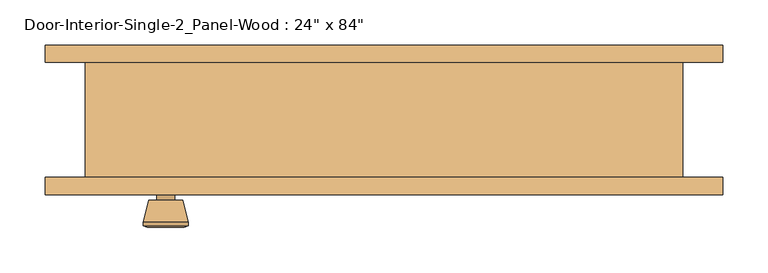
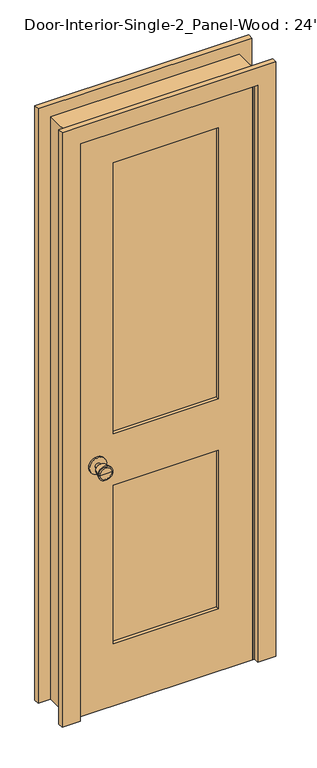
"""IFC4 building model written with IfcOpenShell, lengths in millimetres: door geometry."""

from ifc_helpers import new_model, si_unit, point, frame, frame_2d, origin, place, context, project, spatial, polyline, circle_curve, trimmed, segment, composite_curve, outline, extrude, faceted_brep, source, transform, mapped, element, save
from ifc_brep_helpers import plane_surface, cylinder_surface, revolved_surface, advanced_brep


def door_e337afa5(model_context):
    return source(origin(), model_context, "Body", "SolidModel", [
        advanced_brep(
        [(-241.3, -19.4, 914.4), (-251.3, -19.4, 914.4), (-231.3, -19.4, 914.4), (-220.8241324, 29.6, 914.4), (-261.7758676, 29.6, 914.4), (-241.3, 29.6, 914.4), (-216.3, 27.7721319, 914.4), (-266.3, 27.7721319, 914.4), (-216.3, 24.3084537, 914.4), (-266.3, 24.3084537, 914.4), (-222.663764, -0.4, 914.4), (-259.936236, -0.4, 914.4), (-231.3, -0.4, 914.4), (-251.3, -0.4, 914.4)],
        [
            (0, 1),
            (1, 2, circle_curve(frame((-241.3, -19.4, 914.4), z_axis=(0.0, -1.0, 0.0), x_axis=(-1.0, 0.0, 0.0)), 10.0)),
            (2, 0),
            (2, 1, circle_curve(frame((-241.3, -19.4, 914.4), z_axis=(0.0, -1.0, 0.0), x_axis=(-1.0, 0.0, 0.0)), 10.0)),
            (3, 4, circle_curve(frame((-241.3, 29.6, 914.4), z_axis=(0.0, 1.0, 0.0), x_axis=(-1.0, 0.0, 0.0)), 20.4758676)),
            (4, 5),
            (5, 3),
            (4, 3, circle_curve(frame((-241.3, 29.6, 914.4), z_axis=(0.0, 1.0, 0.0), x_axis=(-1.0, 0.0, 0.0)), 20.4758676)),
            (6, 7, circle_curve(frame((-241.3, 27.7721319, 914.4), z_axis=(0.0, 1.0, 0.0), x_axis=(-1.0, 0.0, 0.0)), 25.0)),
            (7, 4),
            (3, 6),
            (7, 6, circle_curve(frame((-241.3, 27.7721319, 914.4), z_axis=(0.0, 1.0, 0.0), x_axis=(-1.0, 0.0, 0.0)), 25.0)),
            (8, 9, circle_curve(frame((-241.3, 24.3084537, 914.4), z_axis=(0.0, 1.0, 0.0), x_axis=(-1.0, 0.0, 0.0)), 25.0)),
            (9, 7),
            (6, 8),
            (9, 8, circle_curve(frame((-241.3, 24.3084537, 914.4), z_axis=(0.0, 1.0, 0.0), x_axis=(-1.0, 0.0, 0.0)), 25.0)),
            (10, 11, circle_curve(frame((-241.3, -0.4, 914.4), z_axis=(0.0, 1.0, 0.0), x_axis=(-1.0, 0.0, 0.0)), 18.636236)),
            (11, 9),
            (8, 10),
            (11, 10, circle_curve(frame((-241.3, -0.4, 914.4), z_axis=(0.0, 1.0, 0.0), x_axis=(-1.0, 0.0, 0.0)), 18.636236)),
            (12, 13, circle_curve(frame((-241.3, -0.4, 914.4), z_axis=(0.0, 1.0, 0.0), x_axis=(-1.0, 0.0, 0.0)), 10.0)),
            (13, 11),
            (10, 12),
            (13, 12, circle_curve(frame((-241.3, -0.4, 914.4), z_axis=(0.0, 1.0, 0.0), x_axis=(-1.0, 0.0, 0.0)), 10.0)),
            (1, 13),
            (12, 2),
        ],
        [
            plane_surface(frame((-241.3, -19.4, 914.4), z_axis=(0.0, -1.0, 0.0), x_axis=(-1.0, 0.0, 0.0))),
            plane_surface(frame((-241.3, 29.6, 914.4), z_axis=(0.0, 1.0, 0.0), x_axis=(-1.0, 0.0, 0.0))),
            revolved_surface(polyline([(-261.7758676, 29.6, 914.4), (-266.3, 27.7721319, 914.4)]), (-241.3, -19.4, 914.4), (0.0, -1.0, 0.0)),
            cylinder_surface(frame((-241.3, -19.4, 914.4), z_axis=(0.0, -1.0, 0.0), x_axis=(-1.0, 0.0, 0.0)), 25.0),
            revolved_surface(polyline([(-266.3, 24.3084537, 914.4), (-259.936236, -0.4, 914.4)]), (-241.3, -19.4, 914.4), (0.0, -1.0, 0.0)),
            plane_surface(frame((-241.3, -0.4, 914.4), z_axis=(0.0, -1.0, 0.0), x_axis=(-1.0, 0.0, 0.0))),
            cylinder_surface(frame((-241.3, -19.4, 914.4), z_axis=(0.0, -1.0, 0.0), x_axis=(-1.0, 0.0, 0.0)), 10.0),
        ],
        [
            (0, [[1, 2, 3]]),
            (0, [[-3, 4, -1]]),
            (1, [[5, 6, 7]]),
            (1, [[8, -7, -6]]),
            (2, [[9, 10, -5, 11]]),
            (2, [[12, -11, -8, -10]]),
            (3, [[13, 14, -9, 15]]),
            (3, [[16, -15, -12, -14]]),
            (4, [[17, 18, -13, 19]]),
            (4, [[20, -19, -16, -18]]),
            (5, [[21, 22, -17, 23]]),
            (5, [[24, -23, -20, -22]]),
            (6, [[-2, 25, -21, 26]]),
            (6, [[-4, -26, -24, -25]]),
        ],
    ),
        extrude(outline(composite_curve([segment(trimmed(circle_curve(frame_2d((914.4, -241.3)), 30.0), [point((914.4, -271.3))], [point((914.4, -211.3))], False, "CARTESIAN"), True, "CONTINUOUS"), segment(trimmed(circle_curve(frame_2d((914.4, -241.3)), 30.0), [point((914.4, -211.3))], [point((914.4, -271.3))], False, "CARTESIAN"), True, "CONTINUOUS")], self_intersect=False)), frame((0.0, -25.4, 0.0), z_axis=(0.0, 1.0, 0.0), x_axis=(0.0, 0.0, 1.0)), (0.0, 0.0, 1.0), 6.0),
        advanced_brep(
        [(-241.3, -66.325, 914.4), (-231.3, -66.325, 914.4), (-251.3, -66.325, 914.4), (-220.8241324, -115.325, 914.4), (-241.3, -115.325, 914.4), (-261.7758676, -115.325, 914.4), (-216.3, -113.4971319, 914.4), (-266.3, -113.4971319, 914.4), (-216.3, -110.0334537, 914.4), (-266.3, -110.0334537, 914.4), (-222.663764, -85.325, 914.4), (-259.936236, -85.325, 914.4), (-231.3, -85.325, 914.4), (-251.3, -85.325, 914.4)],
        [
            (0, 1),
            (1, 2, circle_curve(frame((-241.3, -66.325, 914.4), z_axis=(0.0, 1.0, 0.0), x_axis=(-1.0, 0.0, 0.0)), 10.0)),
            (2, 0),
            (2, 1, circle_curve(frame((-241.3, -66.325, 914.4), z_axis=(0.0, 1.0, 0.0), x_axis=(-1.0, 0.0, 0.0)), 10.0)),
            (3, 4),
            (4, 5),
            (5, 3, circle_curve(frame((-241.3, -115.325, 914.4), z_axis=(0.0, -1.0, 0.0), x_axis=(-1.0, 0.0, 0.0)), 20.4758676)),
            (3, 5, circle_curve(frame((-241.3, -115.325, 914.4), z_axis=(0.0, -1.0, 0.0), x_axis=(-1.0, 0.0, 0.0)), 20.4758676)),
            (6, 3),
            (5, 7),
            (7, 6, circle_curve(frame((-241.3, -113.4971319, 914.4), z_axis=(0.0, -1.0, 0.0), x_axis=(-1.0, 0.0, 0.0)), 25.0)),
            (6, 7, circle_curve(frame((-241.3, -113.4971319, 914.4), z_axis=(0.0, -1.0, 0.0), x_axis=(-1.0, 0.0, 0.0)), 25.0)),
            (8, 6),
            (7, 9),
            (9, 8, circle_curve(frame((-241.3, -110.0334537, 914.4), z_axis=(0.0, -1.0, 0.0), x_axis=(-1.0, 0.0, 0.0)), 25.0)),
            (8, 9, circle_curve(frame((-241.3, -110.0334537, 914.4), z_axis=(0.0, -1.0, 0.0), x_axis=(-1.0, 0.0, 0.0)), 25.0)),
            (10, 8),
            (9, 11),
            (11, 10, circle_curve(frame((-241.3, -85.325, 914.4), z_axis=(0.0, -1.0, 0.0), x_axis=(-1.0, 0.0, 0.0)), 18.636236)),
            (10, 11, circle_curve(frame((-241.3, -85.325, 914.4), z_axis=(0.0, -1.0, 0.0), x_axis=(-1.0, 0.0, 0.0)), 18.636236)),
            (12, 10),
            (11, 13),
            (13, 12, circle_curve(frame((-241.3, -85.325, 914.4), z_axis=(0.0, -1.0, 0.0), x_axis=(-1.0, 0.0, 0.0)), 10.0)),
            (12, 13, circle_curve(frame((-241.3, -85.325, 914.4), z_axis=(0.0, -1.0, 0.0), x_axis=(-1.0, 0.0, 0.0)), 10.0)),
            (1, 12),
            (13, 2),
        ],
        [
            plane_surface(frame((-241.3, -66.325, 914.4), z_axis=(0.0, 1.0, 0.0), x_axis=(-1.0, 0.0, 0.0))),
            plane_surface(frame((-241.3, -115.325, 914.4), z_axis=(0.0, -1.0, 0.0), x_axis=(-1.0, 0.0, 0.0))),
            revolved_surface(polyline([(-261.7758676, -115.325, 914.4), (-266.3, -113.4971319, 914.4)]), (-241.3, -66.325, 914.4), (0.0, 1.0, 0.0)),
            cylinder_surface(frame((-241.3, -66.325, 914.4), z_axis=(0.0, 1.0, 0.0), x_axis=(-1.0, 0.0, 0.0)), 25.0),
            revolved_surface(polyline([(-266.3, -110.0334537, 914.4), (-259.936236, -85.325, 914.4)]), (-241.3, -66.325, 914.4), (0.0, 1.0, 0.0)),
            plane_surface(frame((-241.3, -85.325, 914.4), z_axis=(0.0, 1.0, 0.0), x_axis=(-1.0, 0.0, 0.0))),
            cylinder_surface(frame((-241.3, -66.325, 914.4), z_axis=(0.0, 1.0, 0.0), x_axis=(-1.0, 0.0, 0.0)), 10.0),
        ],
        [
            (0, [[1, 2, 3]]),
            (0, [[-3, 4, -1]]),
            (1, [[5, 6, 7]]),
            (1, [[-6, -5, 8]]),
            (2, [[9, -7, 10, 11]]),
            (2, [[-10, -8, -9, 12]]),
            (3, [[13, -11, 14, 15]]),
            (3, [[-14, -12, -13, 16]]),
            (4, [[17, -15, 18, 19]]),
            (4, [[-18, -16, -17, 20]]),
            (5, [[21, -19, 22, 23]]),
            (5, [[-22, -20, -21, 24]]),
            (6, [[25, -23, 26, -2]]),
            (6, [[-26, -24, -25, -4]]),
        ],
    ),
        extrude(outline(composite_curve([segment(trimmed(circle_curve(frame_2d((914.4, -241.3)), 30.0), [point((914.4, -271.3))], [point((914.4, -211.3))], False, "CARTESIAN"), True, "CONTINUOUS"), segment(trimmed(circle_curve(frame_2d((914.4, -241.3)), 30.0), [point((914.4, -211.3))], [point((914.4, -271.3))], False, "CARTESIAN"), True, "CONTINUOUS")], self_intersect=False)), frame((0.0, -66.325, 0.0), z_axis=(0.0, 1.0, 0.0), x_axis=(0.0, 0.0, 1.0)), (0.0, 0.0, 1.0), 6.0),
        faceted_brep([(330.2, -60.325, 0.0), (304.8, -60.325, 0.0), (304.8, -25.4, 0.0), (292.1, -25.4, 0.0), (292.1, 9.525, 0.0), (304.8, 9.525, 0.0), (304.8, 66.675, 0.0), (330.2, 66.675, 0.0), (330.2, 66.675, 2159.0), (330.2, -60.325, 2159.0), (304.8, 66.675, 2133.6), (-304.8, 66.675, 2133.6), (-304.8, 66.675, 0.0), (-330.2, 66.675, 0.0), (-330.2, 66.675, 2159.0), (304.8, 9.525, 2133.6), (292.1, 9.525, 2120.9), (-292.1, 9.525, 2120.9), (-292.1, 9.525, 0.0), (-304.8, 9.525, 0.0), (-304.8, 9.525, 2133.6), (292.1, -25.4, 2120.9), (304.8, -25.4, 2133.6), (-304.8, -25.4, 2133.6), (-304.8, -25.4, 0.0), (-292.1, -25.4, 0.0), (-292.1, -25.4, 2120.9), (304.8, -60.325, 2133.6), (-330.2, -60.325, 2159.0), (-330.2, -60.325, 0.0), (-304.8, -60.325, 0.0), (-304.8, -60.325, 2133.6)], [[[0, 1, 2, 3, 4, 5, 6, 7]], [[7, 8, 9, 0]], [[6, 10, 11, 12, 13, 14, 8, 7]], [[5, 15, 10, 6]], [[4, 16, 17, 18, 19, 20, 15, 5]], [[3, 21, 16, 4]], [[2, 22, 23, 24, 25, 26, 21, 3]], [[1, 27, 22, 2]], [[0, 9, 28, 29, 30, 31, 27, 1]], [[8, 14, 28, 9]], [[15, 20, 11, 10]], [[21, 26, 17, 16]], [[27, 31, 23, 22]], [[29, 13, 12, 19, 18, 25, 24, 30]], [[14, 13, 29, 28]], [[20, 19, 12, 11]], [[26, 25, 18, 17]], [[31, 30, 24, 23]]]),
        extrude(outline(polyline([(2133.6, -304.8), (0.0, -304.8), (0.0, 304.8), (2133.6, 304.8), (2133.6, -304.8)]), holes=[polyline([(2014.5375, -184.15), (2014.5375, 184.15), (1009.65, 184.15), (1009.65, -184.15), (2014.5375, -184.15)]), polyline([(819.15, -184.15), (819.15, 184.15), (231.775, 184.15), (231.775, -184.15), (819.15, -184.15)])]), frame((0.0, -60.325, 0.0), z_axis=(0.0, 1.0, 0.0), x_axis=(0.0, 0.0, 1.0)), (0.0, 0.0, 1.0), 34.925),
        extrude(outline(polyline([(184.15, -37.0416667), (184.15, -48.6833333), (-184.15, -48.6833333), (-184.15, -37.0416667), (184.15, -37.0416667)])), frame((0.0, 0.0, 1009.65), z_axis=(0.0, 0.0, 1.0), x_axis=(1.0, 0.0, 0.0)), (0.0, 0.0, 1.0), 1004.8875),
        extrude(outline(polyline([(184.15, -37.0416667), (184.15, -48.6833333), (-184.15, -48.6833333), (-184.15, -37.0416667), (184.15, -37.0416667)])), frame((0.0, 0.0, 231.775), z_axis=(0.0, 0.0, 1.0), x_axis=(1.0, 0.0, 0.0)), (0.0, 0.0, 1.0), 587.375),
        extrude(outline(polyline([(0.0, 374.65), (2203.45, 374.65), (2203.45, -374.65), (0.0, -374.65), (0.0, -311.15), (2139.95, -311.15), (2139.95, 311.15), (0.0, 311.15), (0.0, 374.65)])), frame((0.0, -79.375, 0.0), z_axis=(0.0, 1.0, 0.0), x_axis=(0.0, 0.0, 1.0)), (0.0, 0.0, 1.0), 19.05),
        extrude(outline(polyline([(0.0, 374.65), (2203.45, 374.65), (2203.45, -374.65), (0.0, -374.65), (0.0, -311.15), (2139.95, -311.15), (2139.95, 311.15), (0.0, 311.15), (0.0, 374.65)])), frame((0.0, 66.675, 0.0), z_axis=(0.0, 1.0, 0.0), x_axis=(0.0, 0.0, 1.0)), (0.0, 0.0, 1.0), 19.05),
    ])


if __name__ == "__main__":
    model = new_model("IFC4")
    model_context = context("Model", 3, world=origin())
    ifc_project = project(units=[si_unit("LENGTHUNIT", "METRE", prefix="MILLI")], contexts=[model_context])
    site = spatial("IfcSite", under=ifc_project)
    building = spatial("IfcBuilding", under=site)
    placement = place(None, origin())
    door_shape = door_e337afa5(model_context)
    element("IfcDoor", 1, ObjectType="Door-Interior-Single-2_Panel-Wood : 24\" x 84\"", at=placement, inside=building, context=model_context, shape_type="MappedRepresentation", body=[
        mapped(door_shape, transform((0.0, 0.0, 0.0), x_axis=(1.0, 0.0, 0.0), y_axis=(0.0, 1.0, 0.0), z_axis=(0.0, 0.0, 1.0))),
    ])
    save(model, "model.ifc")

# Revit data of these elements
# Type "Door-Interior-Single-2_Panel-Wood : 24\" x 84\""
#   Type Mark = "10"
#   Assembly Code = "C1020300"
#   Analytic Construction = "Wooden"
#   Top Rail = 0' - 4 11/16"
#   Thickness = 0' - 1 3/8"
#   Thermal Resistance (R) = 2.5876 (h·ft²·°F)/BTU
#   Swing Angle [instance default] = 90.00°
#   Stiles = 0' - 4 3/4"
#   Rough Width = 2' - 2"
#   Rough Height = 7' - 1"
#   Lock Rail = 0' - 7 1/2"
#   Height = 7' - 0"
#   Width = 2' - 0"
#   Heat Transfer Coefficient (U) = 0.3865 BTU/(h·ft²·°F)
#   Bottom Rail = 0' - 9 1/8"
#   Trim Material = Cherry
#   Panel Material = Cherry
#   Frame Material = Cherry
#   Door Handle Material = Aluminum
#   Visual Light Transmittance = 0
#   Solar Heat Gain Coefficient = 0
#   Wall Closure = (empty or 0)
#   Function = (empty or 0)
# Element 1 (IfcDoor, "Door-Interior-Single-2_Panel-Wood : 24\" x 84\"")
#   Materials on its faces: "Cherry", "Aluminum"
# Materials
#   "Cherry": class "Wood", colour RGB 226 177 128, transparency 0, Description = "Prunus Serotina", Cost = 0
#   "Aluminum": class "Metal", colour RGB 247 247 247, transparency 0, Description = "Aluminum 6061", Cost = 0
